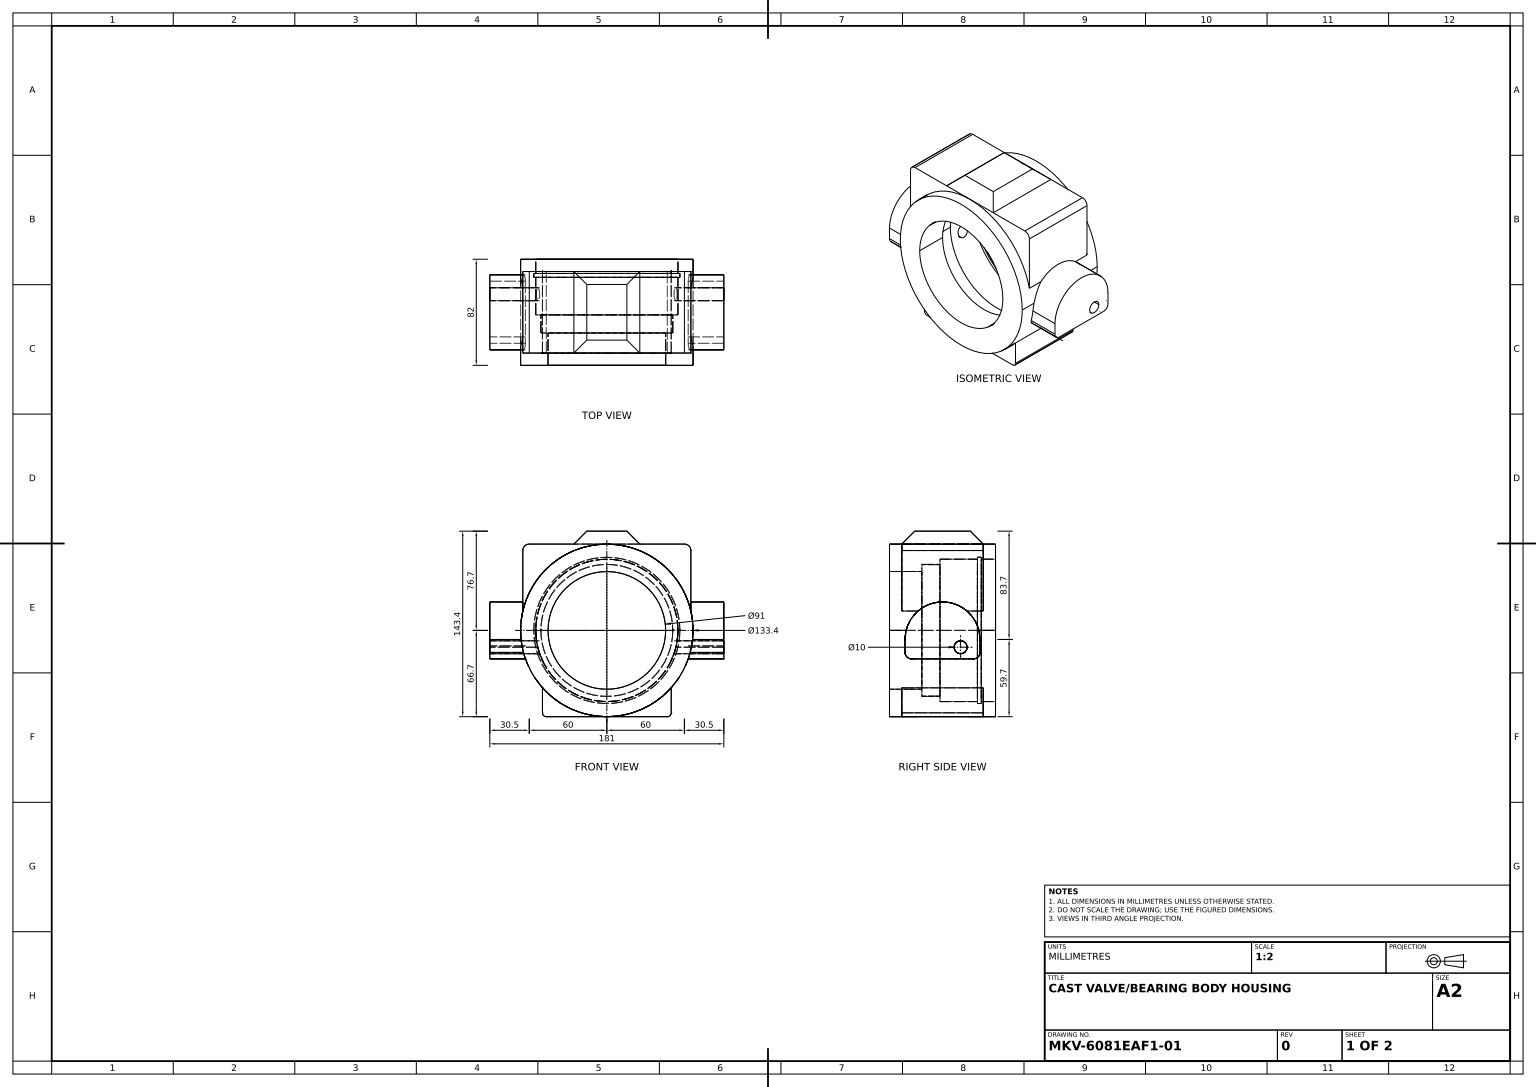
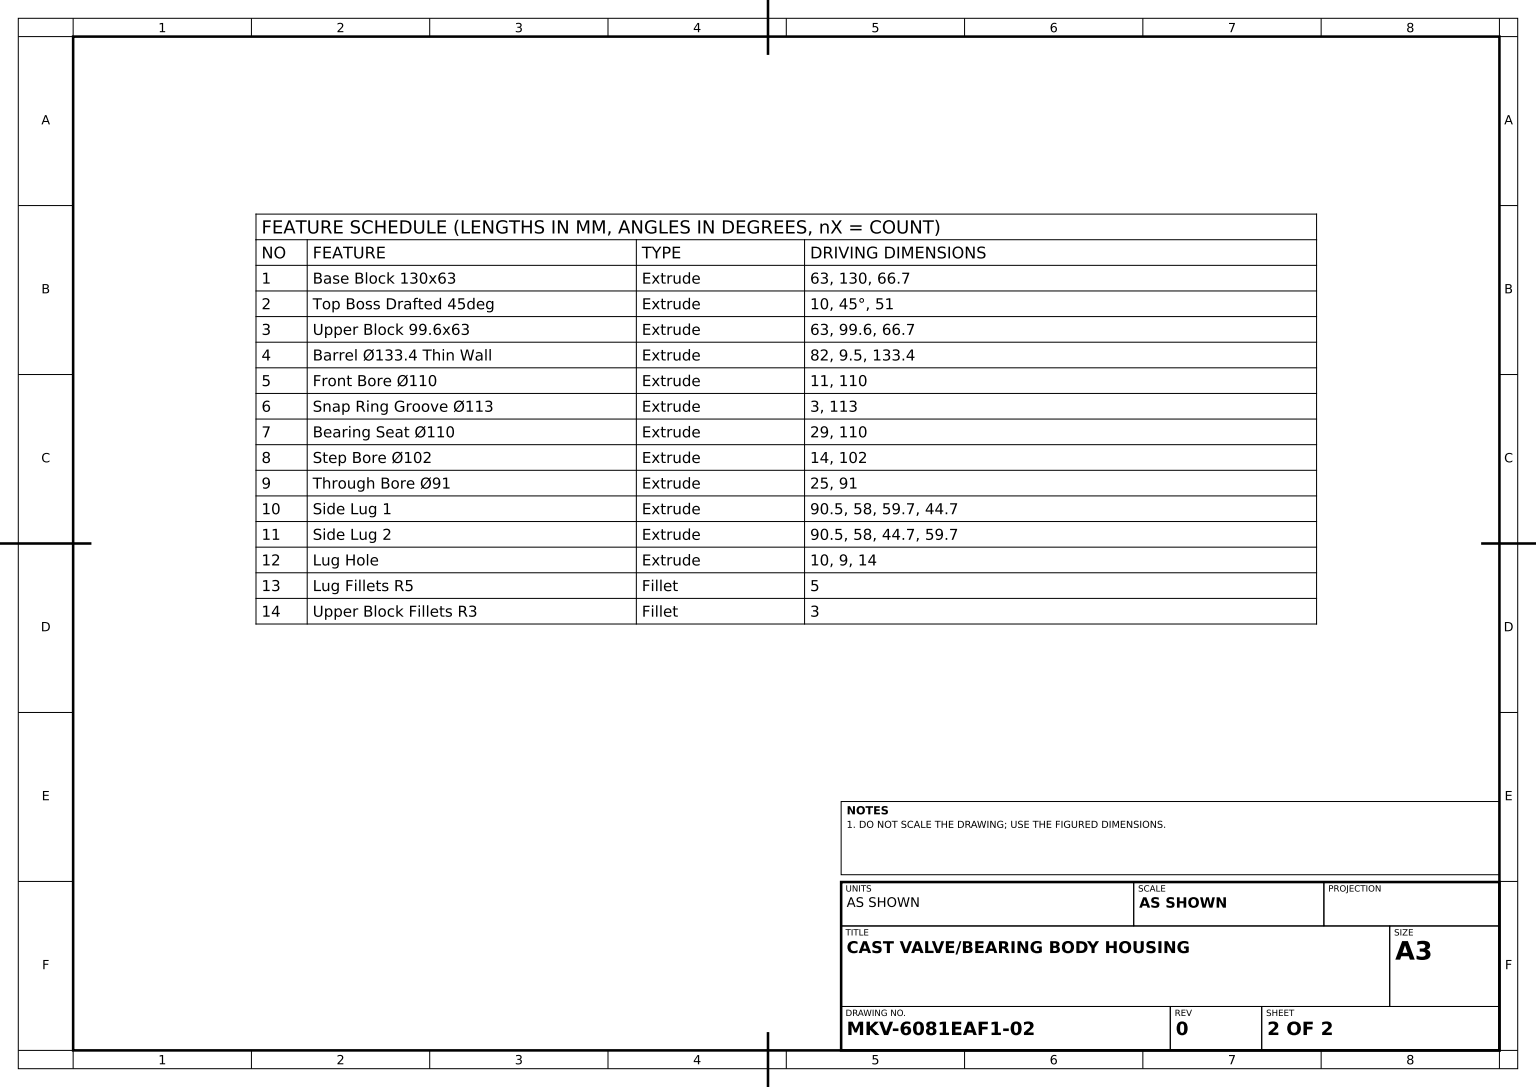
from build123d import *

# Parameters (mm, degrees)
BASE_BLOCK_SKETCH_W           = 130
BASE_BLOCK_SKETCH_H           = 66.7
BASE_BLOCK_130X63_DEPTH       = 31.5
TOP_BOSS_SKETCH_W             = 51
TOP_BOSS_SKETCH_H             = 63
TOP_BOSS_DRAFTED_45DEG_DEPTH  = 10
TOP_BOSS_DRAFTED_45DEG_TAPER  = 45
UPPER_BLOCK_SKETCH_W          = 99.6
UPPER_BLOCK_SKETCH_H          = 66.7
UPPER_BLOCK_99_6X63_DEPTH     = 31.5
BARREL_START                  = 9.5
BARREL_SKETCH_133_4_R         = 66.7
BARREL_133_4_THIN_WALL_DEPTH  = 82
FRONT_BORE_SKETCH_110_R       = 55
FRONT_BORE_110_DEPTH          = 11
SNAP_RING_GROOVE_SKETCH_113_R = 56.5
SNAP_RING_GROOVE_113_DEPTH    = 3
BEARING_SEAT_SKETCH_110_R     = 55
BEARING_SEAT_110_DEPTH        = 29
STEP_BORE_SKETCH_102_R        = 51
STEP_BORE_102_DEPTH           = 14
THROUGH_BORE_SKETCH_91_R      = 45.5
THROUGH_BORE_91_DEPTH         = 25
SIDE_LUG_1_REACH              = 192.795
SIDE_LUG_2_REACH              = 212.836
LUG_HOLE_SKETCH_R             = 5
LUG_HOLE_DEPTH                = 211.836435571
LUG_FILLETS_R5_R              = 5
UPPER_BLOCK_FILLETS_R3_R      = 3


with BuildPart() as part:
    # Base Block Sketch → Base Block 130x63 (new, symmetric)
    with BuildSketch(Plane.XY):
        Rectangle(BASE_BLOCK_SKETCH_W, BASE_BLOCK_SKETCH_H)
    extrude(amount=BASE_BLOCK_130X63_DEPTH, both=True)

    # Top Boss Sketch → Top Boss Drafted 45deg (add)
    with BuildSketch(Plane(origin=(0, 33.35, 0), x_dir=(1, 0, 0), z_dir=(0, 1, 0))):
        Rectangle(TOP_BOSS_SKETCH_W, TOP_BOSS_SKETCH_H)
    extrude(amount=TOP_BOSS_DRAFTED_45DEG_DEPTH, taper=TOP_BOSS_DRAFTED_45DEG_TAPER)

    # Upper Block Sketch → Upper Block 99.6x63 (add, symmetric)
    with BuildSketch(Plane.XY):
        with Locations((0, -66.7)):
            Rectangle(UPPER_BLOCK_SKETCH_W, UPPER_BLOCK_SKETCH_H)
    extrude(amount=UPPER_BLOCK_99_6X63_DEPTH, both=True)

    # Barrel Sketch Ø133.4 → Barrel Ø133.4 Thin Wall (add)
    with BuildSketch(Plane.XY.offset(31.5).offset(BARREL_START)):
        with Locations((0, -33.35)):
            Circle(BARREL_SKETCH_133_4_R)
    extrude(amount=-BARREL_133_4_THIN_WALL_DEPTH)

    # Front Bore Sketch Ø110 → Front Bore Ø110 (cut)
    with BuildSketch(Plane(origin=(0, 0, -41), x_dir=(-1, 0, 0), z_dir=(0, 0, -1))):
        with Locations((0, -33.35)):
            Circle(FRONT_BORE_SKETCH_110_R)
    extrude(amount=-FRONT_BORE_110_DEPTH, mode=Mode.SUBTRACT)

    # Snap Ring Groove Sketch Ø113 → Snap Ring Groove Ø113 (cut)
    with BuildSketch(Plane(origin=(0, 0, -30), x_dir=(-1, 0, 0), z_dir=(0, 0, -1))):
        with Locations((0, -33.35)):
            Circle(SNAP_RING_GROOVE_SKETCH_113_R)
    extrude(amount=-SNAP_RING_GROOVE_113_DEPTH, mode=Mode.SUBTRACT)

    # Bearing Seat Sketch Ø110 → Bearing Seat Ø110 (cut)
    with BuildSketch(Plane(origin=(0, 0, -27), x_dir=(-1, 0, 0), z_dir=(0, 0, -1))):
        with Locations((0, -33.35)):
            Circle(BEARING_SEAT_SKETCH_110_R)
    extrude(amount=-BEARING_SEAT_110_DEPTH, mode=Mode.SUBTRACT)

    # Step Bore Sketch Ø102 → Step Bore Ø102 (cut)
    with BuildSketch(Plane(origin=(0, 0, 2), x_dir=(-1, 0, 0), z_dir=(0, 0, -1))):
        with Locations((0, -33.35)):
            Circle(STEP_BORE_SKETCH_102_R)
    extrude(amount=-STEP_BORE_102_DEPTH, mode=Mode.SUBTRACT)

    # Through Bore Sketch Ø91 → Through Bore Ø91 (cut)
    with BuildSketch(Plane(origin=(0, 0, 16), x_dir=(-1, 0, 0), z_dir=(0, 0, -1))):
        with Locations((0, -33.35)):
            Circle(THROUGH_BORE_SKETCH_91_R)
    extrude(amount=-THROUGH_BORE_91_DEPTH, mode=Mode.SUBTRACT)

    # Side Lug 1 Sketch → Side Lug 1 (add, up to next)
    with BuildSketch(Plane(origin=(90.5, 0, 0), x_dir=(0, 0, -1), z_dir=(1, 0, 0)), mode=Mode.PRIVATE) as side_lug_1_sk1:
        with BuildLine():
            Line((-29, -40.35), (-29, -55.35))
            Line((-29, -55.35), (29, -55.35))
            Line((29, -55.35), (29, -40.35))
            ThreePointArc((29, -40.35), (0, -11.35), (-29, -40.35))
        make_face()
    side_lug_1_tool1 = extrude(side_lug_1_sk1.sketch, amount=-SIDE_LUG_1_REACH, mode=Mode.PRIVATE) - part.part
    add(side_lug_1_tool1.solids().sort_by_distance((90.5, -35.907208, 0))[0])

    # Side Lug 2 Sketch → Side Lug 2 (add, up to next)
    with BuildSketch(Plane(origin=(-90.5, 0, 0), x_dir=(0, 0, -1), z_dir=(1, 0, 0)), mode=Mode.PRIVATE) as side_lug_2_sk1:
        with BuildLine():
            Line((29, -55.35), (-29, -55.35))
            Line((-29, -55.35), (-29, -40.35))
            ThreePointArc((-29, -40.35), (0, -11.35), (29, -40.35))
            Line((29, -40.35), (29, -55.35))
        make_face()
    side_lug_2_tool1 = extrude(side_lug_2_sk1.sketch, amount=SIDE_LUG_2_REACH, mode=Mode.PRIVATE) - part.part
    add(side_lug_2_tool1.solids().sort_by_distance((-90.5, -35.907208, 0))[0])

    # Lug Hole Sketch → Lug Hole (cut, through all)
    with BuildSketch(Plane.ZY.offset(90.5)):
        with Locations((-14, -46.35)):
            Circle(LUG_HOLE_SKETCH_R)
    extrude(amount=-LUG_HOLE_DEPTH, mode=Mode.SUBTRACT)

    # Lug Fillets R5
    lug_fillets_r5_edges = [part.edges().sort_by_distance(p)[0] for p in [
        (-76.733686252, -55.35, 29),
        (-76.733686252, -55.35, -29),
        (-65, 33.35, 0),
        (65, 33.35, 0),
        (76.733686252, -55.35, 29),
        (76.733686252, -55.35, -29),
    ]]
    fillet(lug_fillets_r5_edges, radius=LUG_FILLETS_R5_R)

    # Upper Block Fillets R3
    upper_block_fillets_r3_edges = [part.edges().sort_by_distance(p)[0] for p in [
        (-49.8, -100.05, 0),
        (49.8, -100.05, 0),
    ]]
    fillet(upper_block_fillets_r3_edges, radius=UPPER_BLOCK_FILLETS_R3_R)


solid = part.part
